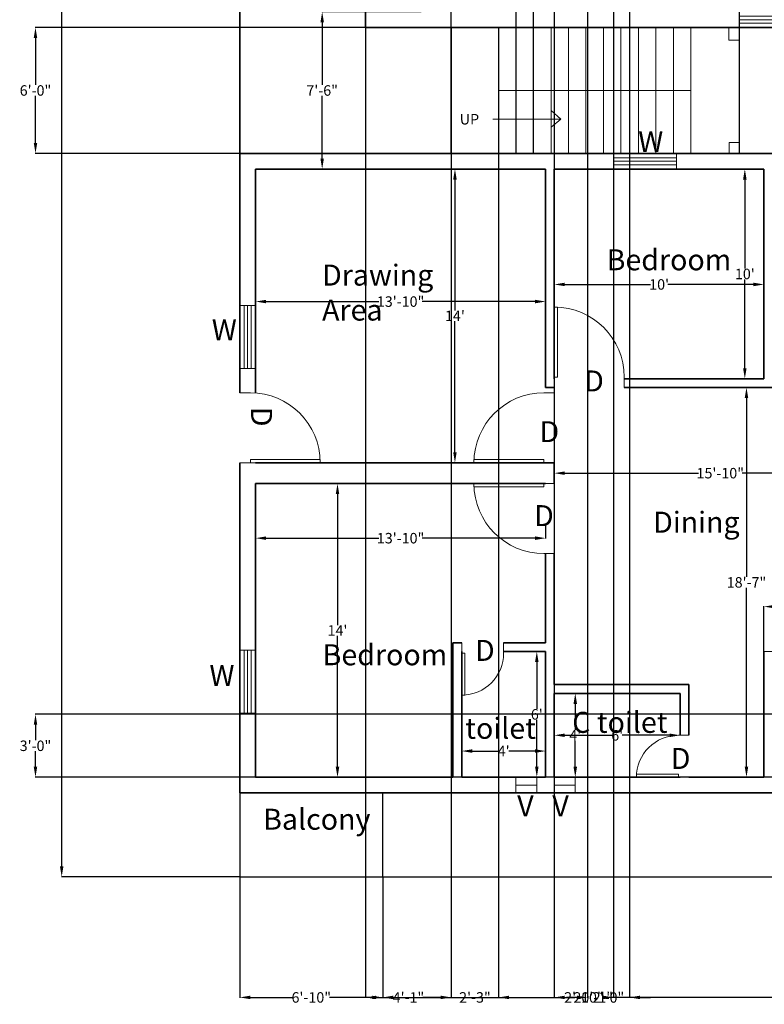
# Model space of a CAD drawing. Units: inches. Extents: x 1936 to 2761, y 1431 to 2889.
# Tile 1 of 6: x 1943 to 2369, y 1436 to 1999. Entities that reach past the tile are written whole.
import ezdxf

# ---------------------------------------------------------------- set-up
doc = ezdxf.new("R2010")
doc.units = ezdxf.units.IN
doc.header["$MEASUREMENT"] = 0
for name, color, linetype, lineweight in [('A-ANNO-DIMS', 172, 'Continuous', 13), ('A-ANNO-SYMB', 50, 'Continuous', 18), ('A-ANNO-TEXT', 50, 'Continuous', 18), ('A-AREA-IDEN', 50, 'Continuous', 18), ('A-FLOR-EDGE', 4, 'Continuous', 25), ('A-FLOR-FIXT', 8, 'Continuous', 18), ('A-GLAZ', 3, 'Continuous', 18), ('A-WALL', 4, 'Continuous', 35), ('doors', 10, 'Continuous', 18), ('stair', 94, 'Continuous', 18)]:
    doc.layers.add(name, color=color, linetype=linetype, lineweight=lineweight)
doc.styles.get("Standard").update_dxf_attribs({"font": 'arial.ttf'})
doc.dimstyles.get("Standard").update_dxf_attribs({"dimtxt": 6, "dimasz": 6, "dimexe": 0.18, "dimexo": 0.0625, "dimgap": 0.09, "dimtad": 0, "dimtih": 1, "dimtoh": 1, "dimdec": 0, "dimzin": 0, "dimdsep": 46, "dimlunit": 3, "dimtxsty": 'Standard', "dimcen": 0.09, "dimadec": 0, "dimazin": 0, "dimtfac": 1, "dimtdec": 0, "dimtofl": 0, "dimtmove": 0, "dimatfit": 3, "dimfxl": 1, "dimtolj": 1, "dimtzin": 0, "dimarcsym": 0})

# ---------------------------------------------------------------- blocks, each defined once
blk = doc.blocks.new('*U4')
for p, q in [((0, 0), (0, 6)), ((24, 0), (24, 6))]:
    blk.add_line(p, q)
blk.add_lwpolyline([(0, 0), (0, -24), (1.75, -24), (1.75, 0)], close=True)
blk.add_arc((0, 0), 24, 270, 0)
blk = doc.blocks.new('*U3')
for p, q in [((0, 0), (0, -6)), ((24, 0), (24, -6))]:
    blk.add_line(p, q)
blk.add_lwpolyline([(0, 0), (0, 24), (1.75, 24), (1.75, 0)], close=True)
blk.add_arc((0, 0), 24, 0, 90)
blk = doc.blocks.new('*U5')
for p, q in [((0, 0), (0, -6)), ((40, 0), (40, -6))]:
    blk.add_line(p, q)
blk.add_lwpolyline([(0, 0), (0, 40), (1.75, 40), (1.75, 0)], close=True)
blk.add_arc((0, 0), 40, 0, 90)
blk = doc.blocks.new('*U2')
for p, q in [((0, 0), (0, 6)), ((40, 0), (40, 6))]:
    blk.add_line(p, q)
blk.add_lwpolyline([(0, 0), (0, -40), (1.75, -40), (1.75, 0)], close=True)
blk.add_arc((0, 0), 40, 270, 360)
blk = doc.blocks.new('*D57')
at = {"layer": 'A-ANNO-DIMS', "color": 0, "lineweight": -2, "transparency": 16777216}
for p, q in [((2078.01, 1709.55), (2078.01, 1702.17)), ((2244.01, 1709.55), (2244.01, 1702.17)), ((2084.01, 1702.35), (2148.56, 1702.35)), ((2238.01, 1702.35), (2173.45, 1702.35))]:
    blk.add_line(p, q, dxfattribs=at)
at = {"layer": 'A-ANNO-DIMS', "color": 0, "transparency": 16777216}
for points in [[(2084.01, 1703.35), (2084.01, 1701.35), (2078.01, 1702.35)], [(2238.01, 1703.35), (2238.01, 1701.35), (2244.01, 1702.35)]]:
    blk.add_solid(points, dxfattribs=at)
at = {"layer": 'Defpoints', "color": 0, "transparency": 16777216}
for p in [(2078.01, 1709.61), (2244.01, 1709.61), (2244.01, 1702.35)]:
    blk.add_point(p, dxfattribs=at)
at = {"layer": 'A-ANNO-DIMS', "color": 0, "transparency": 16777216, "insert": (2161.01, 1702.35), "char_height": 6, "attachment_point": 5}
blk.add_mtext('\\A1;13\'-10"', dxfattribs=at)
blk = doc.blocks.new('*D58')
at = {"layer": 'A-ANNO-DIMS', "color": 0, "lineweight": -2, "transparency": 16777216}
for p, q in [((2124.95, 1733.55), (2125.07, 1733.55)), ((2124.89, 1727.55), (2124.89, 1652.65)), ((2124.89, 1571.55), (2124.89, 1646.45)), ((2124.95, 1565.55), (2125.07, 1565.55))]:
    blk.add_line(p, q, dxfattribs=at)
at = {"layer": 'A-ANNO-DIMS', "color": 0, "transparency": 16777216}
for points in [[(2123.89, 1727.55), (2125.89, 1727.55), (2124.89, 1733.55)], [(2123.89, 1571.55), (2125.89, 1571.55), (2124.89, 1565.55)]]:
    blk.add_solid(points, dxfattribs=at)
at = {"layer": 'Defpoints', "color": 0, "transparency": 16777216}
for p in [(2124.89, 1733.55), (2124.89, 1733.55), (2124.89, 1565.55)]:
    blk.add_point(p, dxfattribs=at)
at = {"layer": 'A-ANNO-DIMS', "color": 0, "transparency": 16777216, "insert": (2124.89, 1649.55), "char_height": 6, "attachment_point": 5}
blk.add_mtext("\\A1;14'", dxfattribs=at)
blk = doc.blocks.new('*D59')
at = {"layer": 'A-ANNO-DIMS', "color": 0, "lineweight": -2, "transparency": 16777216}
for p, q in [((2249.01, 1739.61), (2249.01, 1739.73)), ((2255.01, 1739.55), (2331.56, 1739.55)), ((2433.01, 1739.55), (2356.45, 1739.55)), ((2439.01, 1739.61), (2439.01, 1739.73))]:
    blk.add_line(p, q, dxfattribs=at)
at = {"layer": 'A-ANNO-DIMS', "color": 0, "transparency": 16777216}
for points in [[(2255.01, 1740.55), (2255.01, 1738.55), (2249.01, 1739.55)], [(2433.01, 1740.55), (2433.01, 1738.55), (2439.01, 1739.55)]]:
    blk.add_solid(points, dxfattribs=at)
at = {"layer": 'Defpoints', "color": 0, "transparency": 16777216}
for p in [(2249.01, 1739.55), (2439.01, 1739.55), (2439.01, 1739.55)]:
    blk.add_point(p, dxfattribs=at)
at = {"layer": 'A-ANNO-DIMS', "color": 0, "transparency": 16777216, "insert": (2344.01, 1739.55), "char_height": 6, "attachment_point": 5}
blk.add_mtext('\\A1;15\'-10"', dxfattribs=at)
blk = doc.blocks.new('*D60')
at = {"layer": 'A-ANNO-DIMS', "color": 0, "lineweight": -2, "transparency": 16777216}
for p, q in [((2347.57, 1788.55), (2359.19, 1788.55)), ((2359.01, 1782.55), (2359.01, 1680.2)), ((2359.01, 1571.55), (2359.01, 1673.9)), ((2347.57, 1565.55), (2359.19, 1565.55))]:
    blk.add_line(p, q, dxfattribs=at)
at = {"layer": 'A-ANNO-DIMS', "color": 0, "transparency": 16777216}
for points in [[(2358.01, 1782.55), (2360.01, 1782.55), (2359.01, 1788.55)], [(2358.01, 1571.55), (2360.01, 1571.55), (2359.01, 1565.55)]]:
    blk.add_solid(points, dxfattribs=at)
at = {"layer": 'Defpoints', "color": 0, "transparency": 16777216}
for p in [(2347.51, 1788.55), (2359.01, 1788.55), (2347.51, 1565.55)]:
    blk.add_point(p, dxfattribs=at)
at = {"layer": 'A-ANNO-DIMS', "color": 0, "transparency": 16777216, "insert": (2359.01, 1677.05), "char_height": 6, "attachment_point": 5}
blk.add_mtext('\\A1;18\'-7"', dxfattribs=at)
blk = doc.blocks.new('*D65')
at = {"layer": 'A-ANNO-DIMS', "color": 0, "lineweight": -2, "transparency": 16777216}
for p, q in [((2249.01, 1589.61), (2249.01, 1589.73)), ((2255.01, 1589.55), (2282.14, 1589.55)), ((2315.01, 1589.55), (2287.87, 1589.55)), ((2321.01, 1589.61), (2321.01, 1589.73))]:
    blk.add_line(p, q, dxfattribs=at)
at = {"layer": 'A-ANNO-DIMS', "color": 0, "transparency": 16777216}
for points in [[(2255.01, 1590.55), (2255.01, 1588.55), (2249.01, 1589.55)], [(2315.01, 1590.55), (2315.01, 1588.55), (2321.01, 1589.55)]]:
    blk.add_solid(points, dxfattribs=at)
at = {"layer": 'Defpoints', "color": 0, "transparency": 16777216}
for p in [(2249.01, 1589.55), (2321.01, 1589.55), (2321.01, 1589.55)]:
    blk.add_point(p, dxfattribs=at)
at = {"layer": 'A-ANNO-DIMS', "color": 0, "transparency": 16777216, "insert": (2285.01, 1589.55), "char_height": 6, "attachment_point": 5}
blk.add_mtext("\\A1;6'", dxfattribs=at)
blk = doc.blocks.new('*D66')
at = {"layer": 'A-ANNO-DIMS', "color": 0, "lineweight": -2, "transparency": 16777216}
for p, q in [((2261.07, 1613.55), (2261.19, 1613.55)), ((2261.01, 1607.55), (2261.01, 1592.64)), ((2261.01, 1571.55), (2261.01, 1586.46)), ((2261.07, 1565.55), (2261.19, 1565.55))]:
    blk.add_line(p, q, dxfattribs=at)
at = {"layer": 'A-ANNO-DIMS', "color": 0, "transparency": 16777216}
for points in [[(2260.01, 1607.55), (2262.01, 1607.55), (2261.01, 1613.55)], [(2260.01, 1571.55), (2262.01, 1571.55), (2261.01, 1565.55)]]:
    blk.add_solid(points, dxfattribs=at)
at = {"layer": 'Defpoints', "color": 0, "transparency": 16777216}
for p in [(2261.01, 1613.55), (2261.01, 1613.55), (2261.01, 1565.55)]:
    blk.add_point(p, dxfattribs=at)
at = {"layer": 'A-ANNO-DIMS', "color": 0, "transparency": 16777216, "insert": (2261.01, 1589.55), "char_height": 6, "attachment_point": 5}
blk.add_mtext("\\A1;4'", dxfattribs=at)
blk = doc.blocks.new('*D67')
at = {"layer": 'A-ANNO-DIMS', "color": 0, "lineweight": -2, "transparency": 16777216}
for p, q in [((2234.79, 1637.55), (2239.17, 1637.55)), ((2238.99, 1631.55), (2238.99, 1604.7)), ((2238.99, 1571.55), (2238.99, 1598.4)), ((2234.79, 1565.55), (2239.17, 1565.55))]:
    blk.add_line(p, q, dxfattribs=at)
at = {"layer": 'A-ANNO-DIMS', "color": 0, "transparency": 16777216}
for points in [[(2237.99, 1631.55), (2239.99, 1631.55), (2238.99, 1637.55)], [(2237.99, 1571.55), (2239.99, 1571.55), (2238.99, 1565.55)]]:
    blk.add_solid(points, dxfattribs=at)
at = {"layer": 'Defpoints', "color": 0, "transparency": 16777216}
for p in [(2234.73, 1637.55), (2238.99, 1637.55), (2234.73, 1565.55)]:
    blk.add_point(p, dxfattribs=at)
at = {"layer": 'A-ANNO-DIMS', "color": 0, "transparency": 16777216, "insert": (2238.99, 1601.55), "char_height": 6, "attachment_point": 5}
blk.add_mtext("\\A1;6'", dxfattribs=at)
blk = doc.blocks.new('*D68')
at = {"layer": 'A-ANNO-DIMS', "color": 0, "lineweight": -2, "transparency": 16777216}
for p, q in [((2196.01, 1580.6), (2196.01, 1580.72)), ((2202.01, 1580.54), (2217.03, 1580.54)), ((2238.01, 1580.54), (2222.98, 1580.54)), ((2244.01, 1580.6), (2244.01, 1580.72))]:
    blk.add_line(p, q, dxfattribs=at)
at = {"layer": 'A-ANNO-DIMS', "color": 0, "transparency": 16777216}
for points in [[(2202.01, 1581.54), (2202.01, 1579.54), (2196.01, 1580.54)], [(2238.01, 1581.54), (2238.01, 1579.54), (2244.01, 1580.54)]]:
    blk.add_solid(points, dxfattribs=at)
at = {"layer": 'Defpoints', "color": 0, "transparency": 16777216}
for p in [(2196.01, 1580.54), (2196.01, 1580.54), (2244.01, 1580.54)]:
    blk.add_point(p, dxfattribs=at)
at = {"layer": 'A-ANNO-DIMS', "color": 0, "transparency": 16777216, "insert": (2220.01, 1580.54), "char_height": 6, "attachment_point": 5}
blk.add_mtext("\\A1;4'", dxfattribs=at)
blk = doc.blocks.new('*D69')
at = {"layer": 'A-ANNO-DIMS', "color": 0, "lineweight": -2, "transparency": 16777216}
for p, q in [((2078.01, 1837.81), (2078.01, 1837.93)), ((2084.01, 1837.75), (2148.56, 1837.75)), ((2238.01, 1837.75), (2173.45, 1837.75)), ((2244.01, 1837.81), (2244.01, 1837.93))]:
    blk.add_line(p, q, dxfattribs=at)
at = {"layer": 'A-ANNO-DIMS', "color": 0, "transparency": 16777216}
for points in [[(2084.01, 1838.75), (2084.01, 1836.75), (2078.01, 1837.75)], [(2238.01, 1838.75), (2238.01, 1836.75), (2244.01, 1837.75)]]:
    blk.add_solid(points, dxfattribs=at)
at = {"layer": 'Defpoints', "color": 0, "transparency": 16777216}
for p in [(2078.01, 1837.75), (2244.01, 1837.75), (2244.01, 1837.75)]:
    blk.add_point(p, dxfattribs=at)
at = {"layer": 'A-ANNO-DIMS', "color": 0, "transparency": 16777216, "insert": (2161.01, 1837.75), "char_height": 6, "attachment_point": 5}
blk.add_mtext('\\A1;13\'-10"', dxfattribs=at)
blk = doc.blocks.new('*D70')
at = {"layer": 'A-ANNO-DIMS', "color": 0, "lineweight": -2, "transparency": 16777216}
for p, q in [((2187.65, 1913.55), (2192.3, 1913.55)), ((2192.12, 1907.55), (2192.12, 1832.65)), ((2192.12, 1751.55), (2192.12, 1826.45)), ((2187.65, 1745.55), (2192.3, 1745.55))]:
    blk.add_line(p, q, dxfattribs=at)
at = {"layer": 'A-ANNO-DIMS', "color": 0, "transparency": 16777216}
for points in [[(2191.12, 1907.55), (2193.12, 1907.55), (2192.12, 1913.55)], [(2191.12, 1751.55), (2193.12, 1751.55), (2192.12, 1745.55)]]:
    blk.add_solid(points, dxfattribs=at)
at = {"layer": 'Defpoints', "color": 0, "transparency": 16777216}
for p in [(2187.59, 1913.55), (2192.12, 1913.55), (2187.59, 1745.55)]:
    blk.add_point(p, dxfattribs=at)
at = {"layer": 'A-ANNO-DIMS', "color": 0, "transparency": 16777216, "insert": (2192.12, 1829.55), "char_height": 6, "attachment_point": 5}
blk.add_mtext("\\A1;14'", dxfattribs=at)
blk = doc.blocks.new('*D71')
at = {"layer": 'A-ANNO-DIMS', "color": 0, "lineweight": -2, "transparency": 16777216}
for p, q in [((2249.01, 1853.49), (2249.01, 1847.37)), ((2369.01, 1853.49), (2369.01, 1847.37)), ((2255.01, 1847.55), (2304.11, 1847.55)), ((2363.01, 1847.55), (2313.91, 1847.55))]:
    blk.add_line(p, q, dxfattribs=at)
at = {"layer": 'A-ANNO-DIMS', "color": 0, "transparency": 16777216}
for points in [[(2255.01, 1848.55), (2255.01, 1846.55), (2249.01, 1847.55)], [(2363.01, 1848.55), (2363.01, 1846.55), (2369.01, 1847.55)]]:
    blk.add_solid(points, dxfattribs=at)
at = {"layer": 'Defpoints', "color": 0, "transparency": 16777216}
for p in [(2249.01, 1853.55), (2369.01, 1853.55), (2249.01, 1847.55)]:
    blk.add_point(p, dxfattribs=at)
at = {"layer": 'A-ANNO-DIMS', "color": 0, "transparency": 16777216, "insert": (2309.01, 1847.55), "char_height": 6, "attachment_point": 5}
blk.add_mtext("\\A1;10'", dxfattribs=at)
blk = doc.blocks.new('*D72')
at = {"layer": 'A-ANNO-DIMS', "color": 0, "lineweight": -2, "transparency": 16777216}
for p, q in [((2354.08, 1913.55), (2358.25, 1913.55)), ((2358.07, 1907.55), (2358.07, 1856.7)), ((2358.07, 1799.55), (2358.07, 1850.4)), ((2354.08, 1793.55), (2358.25, 1793.55))]:
    blk.add_line(p, q, dxfattribs=at)
at = {"layer": 'A-ANNO-DIMS', "color": 0, "transparency": 16777216}
for points in [[(2357.07, 1907.55), (2359.07, 1907.55), (2358.07, 1913.55)], [(2357.07, 1799.55), (2359.07, 1799.55), (2358.07, 1793.55)]]:
    blk.add_solid(points, dxfattribs=at)
at = {"layer": 'Defpoints', "color": 0, "transparency": 16777216}
for p in [(2354.02, 1913.55), (2358.07, 1913.55), (2354.02, 1793.55)]:
    blk.add_point(p, dxfattribs=at)
at = {"layer": 'A-ANNO-DIMS', "color": 0, "transparency": 16777216, "insert": (2358.07, 1853.55), "char_height": 6, "attachment_point": 5}
blk.add_mtext("\\A1;10'", dxfattribs=at)
blk = doc.blocks.new('*U55')
for p, q in [((-40, 0), (-40, 6)), ((0, 0), (0, 6))]:
    blk.add_line(p, q)
blk.add_lwpolyline([(0, 0), (0, -40), (-1.75, -40), (-1.75, 0)], close=True)
blk.add_arc((0, 0), 40, 180, 270)
blk = doc.blocks.new('*D76')
at = {"layer": 'A-ANNO-DIMS', "color": 0, "lineweight": -2, "transparency": 16777216}
for p, q in [((2068.94, 2816.55), (1966.82, 2816.55)), ((1967, 2810.55), (1967, 2168.77)), ((1967, 1514.55), (1967, 2156.33)), ((2068.94, 1508.55), (1966.82, 1508.55))]:
    blk.add_line(p, q, dxfattribs=at)
at = {"layer": 'A-ANNO-DIMS', "color": 0, "transparency": 16777216}
for points in [[(1966, 2810.55), (1968, 2810.55), (1967, 2816.55)], [(1966, 1514.55), (1968, 1514.55), (1967, 1508.55)]]:
    blk.add_solid(points, dxfattribs=at)
at = {"layer": 'Defpoints', "color": 0, "transparency": 16777216}
for p in [(2069.01, 2816.55), (1967, 1508.55), (2069.01, 1508.55)]:
    blk.add_point(p, dxfattribs=at)
at = {"layer": 'A-ANNO-DIMS', "color": 0, "transparency": 16777216, "insert": (1967, 2162.55), "char_height": 6, "attachment_point": 5}
blk.add_mtext("\\A1;{\\H2x;109'}", dxfattribs=at)
blk = doc.blocks.new('*D77')
at = {"layer": 'A-ANNO-DIMS', "color": 0, "lineweight": -2, "transparency": 16777216}
for p, q in [((2172.87, 2003.55), (2115.94, 2003.55)), ((2116.12, 1997.55), (2116.12, 1961.7)), ((2116.12, 1919.55), (2116.12, 1955.4)), ((2160.94, 1913.55), (2115.94, 1913.55))]:
    blk.add_line(p, q, dxfattribs=at)
at = {"layer": 'A-ANNO-DIMS', "color": 0, "transparency": 16777216}
for points in [[(2115.12, 1997.55), (2117.12, 1997.55), (2116.12, 2003.55)], [(2115.12, 1919.55), (2117.12, 1919.55), (2116.12, 1913.55)]]:
    blk.add_solid(points, dxfattribs=at)
at = {"layer": 'Defpoints', "color": 0, "transparency": 16777216}
for p in [(2172.93, 2003.55), (2116.12, 1913.55), (2161.01, 1913.55)]:
    blk.add_point(p, dxfattribs=at)
at = {"layer": 'A-ANNO-DIMS', "color": 0, "transparency": 16777216, "insert": (2116.12, 1958.55), "char_height": 6, "attachment_point": 5}
blk.add_mtext('\\A1;7\'-6"', dxfattribs=at)
blk = doc.blocks.new('WIN-36')
for p, q in [((0, 9), (0, 0)), ((36, 6.5), (0, 6.5)), ((36, 9), (36, 0)), ((36, 4.5), (0, 4.5)), ((36, 2.5), (0, 2.5))]:
    blk.add_line(p, q)
blk = doc.blocks.new('VENT-12')
for p, q in [((0, 0), (0, 9)), ((12, 0), (12, 9)), ((0, 4.5), (12, 4.5))]:
    blk.add_line(p, q)
blk = doc.blocks.new('COUNTER-KITCHEN-U')
for p, q in [((41, 36), (41, 0)), ((41, 36), (135, 36)), ((135, 36), (135, 0)), ((0, 0), (41, 0)), ((135, 0), (171, 0))]:
    blk.add_line(p, q)
blk = doc.blocks.new('*D93')
at = {"layer": 'A-ANNO-DIMS', "color": 0, "lineweight": -2, "transparency": 16777216}
for p, q in [((2369.01, 1637.61), (2369.01, 1663.38)), ((2375.01, 1663.2), (2411.95, 1663.2)), ((2534.01, 1663.2), (2497.06, 1663.2)), ((2540.01, 1637.61), (2540.01, 1663.38))]:
    blk.add_line(p, q, dxfattribs=at)
at = {"layer": 'A-ANNO-DIMS', "color": 0, "transparency": 16777216}
for points in [[(2375.01, 1664.2), (2375.01, 1662.2), (2369.01, 1663.2)], [(2534.01, 1664.2), (2534.01, 1662.2), (2540.01, 1663.2)]]:
    blk.add_solid(points, dxfattribs=at)
at = {"layer": 'Defpoints', "color": 0, "transparency": 16777216}
for p in [(2540.01, 1663.2), (2369.01, 1637.55), (2540.01, 1637.55)]:
    blk.add_point(p, dxfattribs=at)
at = {"layer": 'A-ANNO-DIMS', "color": 0, "transparency": 16777216, "insert": (2454.51, 1663.2), "char_height": 6, "attachment_point": 5}
blk.add_mtext('\\A1;COUNTER 14\'-3" TYP.', dxfattribs=at)
blk = doc.blocks.new('*D100')
at = {"layer": 'A-ANNO-DIMS', "color": 0, "lineweight": -2, "transparency": 16777216}
for p, q in [((2069.01, 1508.49), (2069.01, 1439.37)), ((2150.78, 1508.49), (2150.78, 1439.37)), ((2075.01, 1439.55), (2099.48, 1439.55)), ((2144.78, 1439.55), (2120.31, 1439.55))]:
    blk.add_line(p, q, dxfattribs=at)
at = {"layer": 'A-ANNO-DIMS', "color": 0, "transparency": 16777216}
for points in [[(2075.01, 1440.55), (2075.01, 1438.55), (2069.01, 1439.55)], [(2144.78, 1440.55), (2144.78, 1438.55), (2150.78, 1439.55)]]:
    blk.add_solid(points, dxfattribs=at)
at = {"layer": 'Defpoints', "color": 0, "transparency": 16777216}
for p in [(2069.01, 1508.55), (2150.78, 1508.55), (2150.78, 1439.55)]:
    blk.add_point(p, dxfattribs=at)
at = {"layer": 'A-ANNO-DIMS', "color": 0, "transparency": 16777216, "insert": (2109.89, 1439.55), "char_height": 6, "attachment_point": 5}
blk.add_mtext('\\A1;6\'-10"', dxfattribs=at)
blk = doc.blocks.new('*D102')
at = {"layer": 'A-ANNO-DIMS', "color": 0, "lineweight": -2, "transparency": 16777216}
for p, q in [((2150.85, 1556.55), (2738.19, 1556.55)), ((2738.01, 1550.55), (2738.01, 1535.7)), ((2738.01, 1514.55), (2738.01, 1529.4)), ((2150.85, 1508.55), (2738.19, 1508.55))]:
    blk.add_line(p, q, dxfattribs=at)
at = {"layer": 'A-ANNO-DIMS', "color": 0, "transparency": 16777216}
for points in [[(2737.01, 1550.55), (2739.01, 1550.55), (2738.01, 1556.55)], [(2737.01, 1514.55), (2739.01, 1514.55), (2738.01, 1508.55)]]:
    blk.add_solid(points, dxfattribs=at)
at = {"layer": 'Defpoints', "color": 0, "transparency": 16777216}
for p in [(2150.78, 1556.55), (2738.01, 1556.55), (2150.78, 1508.55)]:
    blk.add_point(p, dxfattribs=at)
at = {"layer": 'A-ANNO-DIMS', "color": 0, "transparency": 16777216, "insert": (2738.01, 1532.55), "char_height": 6, "attachment_point": 5}
blk.add_mtext('\\A1;4\'-0"', dxfattribs=at)
blk = doc.blocks.new('*D103')
at = {"layer": 'A-ANNO-DIMS', "color": 0, "lineweight": -2, "transparency": 16777216}
for p, q in [((2150.78, 1508.49), (2150.78, 1439.37)), ((2391.78, 1508.49), (2391.78, 1439.37)), ((2156.78, 1439.55), (2260.84, 1439.55)), ((2385.78, 1439.55), (2281.73, 1439.55))]:
    blk.add_line(p, q, dxfattribs=at)
at = {"layer": 'A-ANNO-DIMS', "color": 0, "transparency": 16777216}
for points in [[(2156.78, 1440.55), (2156.78, 1438.55), (2150.78, 1439.55)], [(2385.78, 1440.55), (2385.78, 1438.55), (2391.78, 1439.55)]]:
    blk.add_solid(points, dxfattribs=at)
at = {"layer": 'Defpoints', "color": 0, "transparency": 16777216}
for p in [(2150.78, 1508.55), (2391.78, 1508.55), (2391.78, 1439.55)]:
    blk.add_point(p, dxfattribs=at)
at = {"layer": 'A-ANNO-DIMS', "color": 0, "transparency": 16777216, "insert": (2271.28, 1439.55), "char_height": 6, "attachment_point": 5}
blk.add_mtext('\\A1;20\'-1"', dxfattribs=at)
blk = doc.blocks.new('*D104')
at = {"layer": 'A-ANNO-DIMS', "color": 0, "lineweight": -2, "transparency": 16777216}
for p, q in [((2190.01, 1922.61), (2190.01, 2885.73)), ((2196.01, 2885.55), (2262.35, 2885.55)), ((2348.92, 2885.55), (2282.58, 2885.55)), ((2354.92, 1922.61), (2354.92, 2885.73))]:
    blk.add_line(p, q, dxfattribs=at)
at = {"layer": 'A-ANNO-DIMS', "color": 0, "transparency": 16777216}
for points in [[(2196.01, 2886.55), (2196.01, 2884.55), (2190.01, 2885.55)], [(2348.92, 2886.55), (2348.92, 2884.55), (2354.92, 2885.55)]]:
    blk.add_solid(points, dxfattribs=at)
at = {"layer": 'Defpoints', "color": 0, "transparency": 16777216}
for p in [(2354.92, 2885.55), (2190.01, 1922.55), (2354.92, 1922.55)]:
    blk.add_point(p, dxfattribs=at)
at = {"layer": 'A-ANNO-DIMS', "color": 0, "transparency": 16777216, "insert": (2272.46, 2885.55), "char_height": 6, "attachment_point": 5}
blk.add_mtext('\\A1;13\'-9"', dxfattribs=at)
blk = doc.blocks.new('*D105')
at = {"layer": 'A-ANNO-DIMS', "color": 0, "lineweight": -2, "transparency": 16777216}
for p, q in [((2189.94, 1994.55), (1951.83, 1994.55)), ((1952.01, 1988.55), (1952.01, 1961.7)), ((1952.01, 1928.55), (1952.01, 1955.4)), ((2189.94, 1922.55), (1951.83, 1922.55))]:
    blk.add_line(p, q, dxfattribs=at)
at = {"layer": 'A-ANNO-DIMS', "color": 0, "transparency": 16777216}
for points in [[(1951.01, 1988.55), (1953.01, 1988.55), (1952.01, 1994.55)], [(1951.01, 1928.55), (1953.01, 1928.55), (1952.01, 1922.55)]]:
    blk.add_solid(points, dxfattribs=at)
at = {"layer": 'Defpoints', "color": 0, "transparency": 16777216}
for p in [(1952.01, 1994.55), (2190.01, 1994.55), (2190.01, 1922.55)]:
    blk.add_point(p, dxfattribs=at)
at = {"layer": 'A-ANNO-DIMS', "color": 0, "transparency": 16777216, "insert": (1952.01, 1958.55), "char_height": 6, "attachment_point": 5}
blk.add_mtext('\\A1;6\'-0"', dxfattribs=at)
blk = doc.blocks.new('*D106')
at = {"layer": 'A-ANNO-DIMS', "color": 0, "lineweight": -2, "transparency": 16777216}
for p, q in [((2141.01, 1994.49), (2141.01, 1439.37)), ((2190.01, 1994.49), (2190.01, 1439.37)), ((2147.01, 1439.55), (2157.32, 1439.55)), ((2184.01, 1439.55), (2173.69, 1439.55))]:
    blk.add_line(p, q, dxfattribs=at)
at = {"layer": 'A-ANNO-DIMS', "color": 0, "transparency": 16777216}
for points in [[(2147.01, 1440.55), (2147.01, 1438.55), (2141.01, 1439.55)], [(2184.01, 1440.55), (2184.01, 1438.55), (2190.01, 1439.55)]]:
    blk.add_solid(points, dxfattribs=at)
at = {"layer": 'Defpoints', "color": 0, "transparency": 16777216}
for p in [(2141.01, 1994.55), (2190.01, 1994.55), (2141.01, 1439.55)]:
    blk.add_point(p, dxfattribs=at)
at = {"layer": 'A-ANNO-DIMS', "color": 0, "transparency": 16777216, "insert": (2165.51, 1439.55), "char_height": 6, "attachment_point": 5}
blk.add_mtext('\\A1;4\'-1"', dxfattribs=at)
blk = doc.blocks.new('*D107')
at = {"layer": 'A-ANNO-DIMS', "color": 0, "lineweight": -2, "transparency": 16777216}
for p, q in [((2221.14, 2885.55), (2215.14, 2885.55)), ((2227.14, 1922.61), (2227.14, 2885.73)), ((2237.14, 1922.61), (2237.14, 2885.73)), ((2243.14, 2885.55), (2249.14, 2885.55))]:
    blk.add_line(p, q, dxfattribs=at)
at = {"layer": 'A-ANNO-DIMS', "color": 0, "transparency": 16777216}
for points in [[(2221.14, 2886.55), (2221.14, 2884.55), (2227.14, 2885.55)], [(2243.14, 2886.55), (2243.14, 2884.55), (2237.14, 2885.55)]]:
    blk.add_solid(points, dxfattribs=at)
at = {"layer": 'Defpoints', "color": 0, "transparency": 16777216}
for p in [(2237.14, 2885.55), (2227.14, 1922.55), (2237.14, 1922.55)]:
    blk.add_point(p, dxfattribs=at)
at = {"layer": 'A-ANNO-DIMS', "color": 0, "transparency": 16777216, "insert": (2259.54, 2885.55), "char_height": 6, "attachment_point": 5}
blk.add_mtext('\\A1;0\'-10"', dxfattribs=at)
blk = doc.blocks.new('*D110')
at = {"layer": 'A-ANNO-DIMS', "color": 0, "lineweight": -2, "transparency": 16777216}
for p, q in [((2268.006183, 2279.486911), (2268.006183, 1439.369411)), ((2292.006183, 2279.486911), (2292.006183, 1439.369411)), ((2262.006183, 1439.549411), (2256.006183, 1439.549411)), ((2298.006183, 1439.549411), (2304.006183, 1439.549411))]:
    blk.add_line(p, q, dxfattribs=at)
at = {"layer": 'A-ANNO-DIMS', "color": 0, "transparency": 16777216}
for points in [[(2262.006183, 1440.549411), (2262.006183, 1438.549411), (2268.006183, 1439.549411)], [(2298.006183, 1440.549411), (2298.006183, 1438.549411), (2292.006183, 1439.549411)]]:
    blk.add_solid(points, dxfattribs=at)
at = {"layer": 'Defpoints', "color": 0, "transparency": 16777216}
for p in [(2268.006183, 2279.549411), (2292.006183, 2279.549411), (2292.006183, 1439.549411)]:
    blk.add_point(p, dxfattribs=at)
at = {"layer": 'A-ANNO-DIMS', "color": 0, "transparency": 16777216, "insert": (2280.006183, 1439.549411), "char_height": 6, "attachment_point": 5}
blk.add_mtext('\\A1;2\'-0"', dxfattribs=at)
blk = doc.blocks.new('*D117')
at = {"layer": 'A-ANNO-DIMS', "color": 0, "lineweight": -2, "transparency": 16777216}
for p, q in [((2409.94, 1601.55), (1951.83, 1601.55)), ((1952.01, 1595.55), (1952.01, 1586.7)), ((1952.01, 1571.55), (1952.01, 1580.39)), ((2373.94, 1565.55), (1951.83, 1565.55))]:
    blk.add_line(p, q, dxfattribs=at)
at = {"layer": 'A-ANNO-DIMS', "color": 0, "transparency": 16777216}
for points in [[(1951.01, 1595.55), (1953.01, 1595.55), (1952.01, 1601.55)], [(1951.01, 1571.55), (1953.01, 1571.55), (1952.01, 1565.55)]]:
    blk.add_solid(points, dxfattribs=at)
at = {"layer": 'Defpoints', "color": 0, "transparency": 16777216}
for p in [(1952.01, 1601.55), (2410.01, 1601.55), (2374.01, 1565.55)]:
    blk.add_point(p, dxfattribs=at)
at = {"layer": 'A-ANNO-DIMS', "color": 0, "transparency": 16777216, "insert": (1952.01, 1583.55), "char_height": 6, "attachment_point": 5}
blk.add_mtext('\\A1;3\'-0"', dxfattribs=at)
blk = doc.blocks.new('*D120')
at = {"layer": 'A-ANNO-DIMS', "color": 0, "lineweight": -2, "transparency": 16777216}
for p, q in [((2249.01, 2459.49), (2249.01, 1439.37)), ((2282.92, 2450.49), (2282.92, 1439.37)), ((2255.01, 1439.55), (2255.52, 1439.55)), ((2276.92, 1439.55), (2276.41, 1439.55))]:
    blk.add_line(p, q, dxfattribs=at)
at = {"layer": 'A-ANNO-DIMS', "color": 0, "transparency": 16777216}
for points in [[(2255.01, 1440.55), (2255.01, 1438.55), (2249.01, 1439.55)], [(2276.92, 1440.55), (2276.92, 1438.55), (2282.92, 1439.55)]]:
    blk.add_solid(points, dxfattribs=at)
at = {"layer": 'Defpoints', "color": 0, "transparency": 16777216}
for p in [(2249.01, 2459.55), (2282.92, 2450.55), (2282.92, 1439.55)]:
    blk.add_point(p, dxfattribs=at)
at = {"layer": 'A-ANNO-DIMS', "color": 0, "transparency": 16777216, "insert": (2265.96, 1439.55), "char_height": 6, "attachment_point": 5}
blk.add_mtext('\\A1;2\'-10"', dxfattribs=at)
blk = doc.blocks.new('*D121')
at = {"layer": 'A-ANNO-DIMS', "color": 0, "lineweight": -2, "transparency": 16777216}
for p, q in [((2190.01, 1994.49), (2190.01, 1439.37)), ((2217.14, 1994.49), (2217.14, 1439.37)), ((2184.01, 1439.55), (2178.01, 1439.55)), ((2223.14, 1439.55), (2229.14, 1439.55))]:
    blk.add_line(p, q, dxfattribs=at)
at = {"layer": 'A-ANNO-DIMS', "color": 0, "transparency": 16777216}
for points in [[(2184.01, 1440.55), (2184.01, 1438.55), (2190.01, 1439.55)], [(2223.14, 1440.55), (2223.14, 1438.55), (2217.14, 1439.55)]]:
    blk.add_solid(points, dxfattribs=at)
at = {"layer": 'Defpoints', "color": 0, "transparency": 16777216}
for p in [(2190.01, 1994.55), (2217.14, 1994.55), (2217.14, 1439.55)]:
    blk.add_point(p, dxfattribs=at)
at = {"layer": 'A-ANNO-DIMS', "color": 0, "transparency": 16777216, "insert": (2203.57, 1439.55), "char_height": 6, "attachment_point": 5}
blk.add_mtext('\\A1;2\'-3"', dxfattribs=at)

msp = doc.modelspace()

# ---------------------------------------------------------------- linework, layer by layer
at = {"layer": 'A-ANNO-SYMB'}
for p, q in [((2252.69, 1942.1), (2247.14, 1947.06)), ((2247.14, 1947.06), (2247.14, 1937.64)), ((2213.74, 1942.1), (2252.69, 1942.1)), ((2247.14, 1937.64), (2252.69, 1942.1))]:
    msp.add_line(p, q, dxfattribs=at)
at = {"layer": 'A-FLOR-EDGE'}
for p, q in [((2069.01, 1556.55), (2069.01, 1508.55)), ((2150.78, 1508.55), (2150.78, 1556.55)), ((2069.01, 1508.55), (2150.78, 1508.55))]:
    msp.add_line(p, q, dxfattribs=at)
at = {"layer": 'A-WALL'}
for p, q in [((2069.01, 1867.87), (2069.01, 2639.55)), ((2141.01, 1994.55), (2141.01, 2131.55)), ((2621.01, 1994.55), (2141.01, 1994.55)), ((2150.01, 1994.55), (2141.01, 1994.55)), ((2549.01, 1922.55), (2069.01, 1922.55)), ((2078.01, 1922.55), (2069.01, 1922.55)), ((2069.01, 1922.55), (2069.01, 1785.55)), ((2244.01, 1913.55), (2078.01, 1913.55)), ((2078.01, 1913.55), (2078.01, 1785.44)), ((2244.01, 1913.55), (2244.01, 1788.55)), ((2369.01, 1913.55), (2249.01, 1913.55)), ((2249.01, 1913.55), (2249.01, 1793.55)), ((2369.01, 1793.55), (2369.01, 1913.55)), ((2369.01, 1793.55), (2289.01, 1793.55)), ((2249.01, 1788.55), (2244.01, 1788.55)), ((2374.01, 1788.55), (2289.01, 1788.55)), ((2069.01, 1745.55), (2069.01, 1556.55)), ((2249.01, 1745.55), (2078.01, 1745.55)), ((2249.01, 1745.55), (2249.01, 1733.55)), ((2078.01, 1733.55), (2078.01, 1565.55)), ((2078.01, 1733.55), (2244.01, 1733.55)), ((2244.01, 1693.55), (2244.01, 1642.55)), ((2249.01, 1693.55), (2249.01, 1618.55)), ((2191.01, 1642.55), (2191.01, 1565.55)), ((2191.01, 1642.55), (2196.01, 1642.55)), ((2220.01, 1642.55), (2244.01, 1642.55)), ((2196.01, 1637.55), (2196.01, 1565.55)), ((2220.01, 1637.55), (2244.01, 1637.55)), ((2244.01, 1637.55), (2244.01, 1565.55)), ((2369.01, 1565.55), (2369.01, 1637.55)), ((2249.01, 1618.55), (2326.01, 1618.55)), ((2326.01, 1618.55), (2326.01, 1589.55)), ((2249.01, 1613.55), (2249.01, 1565.55)), ((2249.01, 1613.55), (2321.01, 1613.55)), ((2321.01, 1613.55), (2321.01, 1589.55)), ((2078.01, 1565.55), (2191.01, 1565.55)), ((2196.01, 1565.55), (2244.01, 1565.55)), ((2249.01, 1565.55), (2321.01, 1565.55)), ((2326.01, 1565.55), (2369.01, 1565.55)), ((2069.01, 1556.55), (2597.01, 1556.55))]:
    msp.add_line(p, q, dxfattribs=at)
at = {"layer": 'doors'}
for p, q in [((2249.01, 1788.55), (2249.01, 1793.55)), ((2289.01, 1788.55), (2289.01, 1793.55)), ((2078.01, 1745.55), (2069.01, 1745.55)), ((2244.01, 1733.55), (2249.01, 1733.55)), ((2244.01, 1693.55), (2249.01, 1693.55)), ((2196.01, 1637.55), (2196.01, 1642.55)), ((2220.01, 1637.55), (2220.01, 1642.55)), ((2326.01, 1589.55), (2321.01, 1589.55)), ((2326.01, 1565.55), (2321.01, 1565.55))]:
    msp.add_line(p, q, dxfattribs=at)
at = {"layer": 'stair'}
for p, q in [((2190.01, 1994.55), (2190.01, 1922.55)), ((2217.14, 1994.55), (2217.14, 1922.55)), ((2227.14, 1994.55), (2227.14, 1922.55)), ((2237.14, 1994.55), (2237.14, 1922.55)), ((2247.14, 1994.55), (2247.14, 1922.55)), ((2257.14, 1994.55), (2257.14, 1922.55)), ((2267.14, 1994.55), (2267.14, 1922.55)), ((2277.14, 1994.55), (2277.14, 1922.55)), ((2287.14, 1994.55), (2287.14, 1922.55)), ((2297.14, 1994.55), (2297.14, 1922.55)), ((2307.14, 1994.55), (2307.14, 1922.55)), ((2317.14, 1994.55), (2317.14, 1922.55)), ((2327.14, 1994.55), (2327.14, 1922.55)), ((2354.92, 1994.55), (2354.92, 1922.55)), ((2327.14, 1958.55), (2217.14, 1958.55)), ((2354.92, 1922.55), (2069.01, 1922.55))]:
    msp.add_line(p, q, dxfattribs=at)
for points in [[(2354.92, 1994.55), (2348.85, 1994.55), (2348.85, 1987.36), (2354.92, 1987.36)], [(2354.92, 1922.55), (2349.1, 1922.55), (2349.1, 1928.72), (2354.92, 1928.72)]]:
    msp.add_lwpolyline(points, close=True, dxfattribs=at)

# ---------------------------------------------------------------- block references
at = {"layer": 'A-FLOR-FIXT', "extrusion": (0, 0, -1), "zscale": -1, "rotation": 180}
msp.add_blockref('COUNTER-KITCHEN-U', (-2369.01, 1637.55), dxfattribs=at)
at = {"layer": 'A-GLAZ'}
for name, p in [('WIN-36', (2354.92, 1994.55)), ('WIN-36', (2282.92, 1913.55)), ('VENT-12', (2227.01, 1556.55))]:
    msp.add_blockref(name, p, dxfattribs=at)
for name, p, rotation in [('WIN-36', (2077.91, 1799.44), 89.99999999999744), ('WIN-36', (2077.91, 1602.21), 89.99999999999763), ('VENT-12', (2261.01, 1565.55), 180)]:
    msp.add_blockref(name, p, dxfattribs=dict(at, rotation=rotation))
at = {"layer": 'doors', "xscale": -1}
for name, p, rotation in [('*U2', (2249.01, 1794.55), 180), ('*U55', (2075.01, 1745.55), 90), ('*U5', (2243.01, 1733.55), 90), ('*U3', (2196.01, 1636.55), 180), ('*U4', (2320.01, 1565.55), 270)]:
    msp.add_blockref(name, p, dxfattribs=dict(at, rotation=rotation))
at = {"layer": 'doors', "rotation": 90.00000000000003}
msp.add_blockref('*U5', (2243.01, 1745.55), dxfattribs=at)

# ---------------------------------------------------------------- texts
at = {"layer": 'A-ANNO-TEXT'}
for s, width, heights, insert, char_height, attachment_point in [('UP', 6.6996, [0], (2194.88, 1945.08), 6, 1), ('W', 7.8209, [0.2], (2297.01, 1923.25), 12, 7), ('W', 7.8209, [0.2], (2052.91, 1815.62), 12, 7), ('D', 28.2371, [0.2], (2266.1, 1786.32), 12, 7), ('D', 28.2371, [0.2], (2240.54, 1757.3), 12, 7), ('D', 28.2371, [0.2], (2237.43, 1709.25), 12, 7), ('D', 28.2371, [0.2], (2203.61, 1632.12), 12, 7), ('W', 7.8209, [0.2], (2051.56, 1617.84), 12, 7), ('D', 28.2371, [0.2], (2315.67, 1570.28), 12, 7), ('V', 13.1151, [0], (2227.76, 1543.19), 12, 7), ('V', 13.1151, [0], (2247.86, 1543.11), 12, 7)]:
    msp.add_mtext_dynamic_manual_height_columns(s, width=width, gutter_width=1, heights=heights, dxfattribs=dict(at, insert=insert, char_height=char_height, attachment_point=attachment_point))
at = {"layer": 'A-ANNO-TEXT', "insert": (2087.4, 1766.22), "char_height": 12, "attachment_point": 3, "rotation": 270}
msp.add_mtext_dynamic_manual_height_columns('D', width=28.2371, gutter_width=1, heights=[0.2], dxfattribs=at)
at = {"layer": 'A-AREA-IDEN', "char_height": 12}
for s, insert, attachment_point in [('Bedroom', (2278.96, 1855.65), 7), ('Drawing Area', (2116.07, 1826.88), 7), ('Dining', (2305.61, 1705.5), 7), ('Bedroom', (2116.37, 1629.62), 7), ('toilet', (2198.01, 1587.55), 7), ('C toilet', (2259.23, 1590.95), 7), ('Balcony', (2082.33, 1547.53), 1)]:
    msp.add_mtext_dynamic_manual_height_columns(s, width=55.7076, gutter_width=1, heights=[0], dxfattribs=dict(at, insert=insert, attachment_point=attachment_point))

# ---------------------------------------------------------------- dimensions: what is measured, and where the dimension line sits
at = {"layer": 'A-ANNO-DIMS'}
for base, p1, p2, override, picture, middle in [((2354.92, 2885.55), (2190.01, 1922.55), (2354.92, 1922.55), {"dimdec": 1, "dimlfac": 1, "dimrnd": 0, "dimzin": 1, "dimdsep": 46, "dimlunit": 4, "dimfrac": 2}, '*D104', (2272.46, 2885.55)), ((2237.14, 2885.55), (2227.14, 1922.55), (2237.14, 1922.55), {"dimdec": 1, "dimlfac": 1, "dimrnd": 0, "dimzin": 1, "dimdsep": 46, "dimlunit": 4, "dimfrac": 2}, '*D107', (2259.54, 2885.55)), ((2282.92, 1439.55), (2249.01, 2459.55), (2282.92, 2450.55), {"dimdec": 1, "dimlfac": 1, "dimrnd": 0, "dimzin": 1, "dimdsep": 46, "dimlunit": 4, "dimfrac": 2}, '*D120', (2265.96, 1439.55)), ((2292.01, 1439.55), (2268.01, 2279.55), (2292.01, 2279.55), {"dimdec": 1, "dimlfac": 1, "dimrnd": 0, "dimzin": 1, "dimdsep": 46, "dimlunit": 4, "dimfrac": 2}, '*D110', (2280.01, 1439.55)), ((2141.01, 1439.55), (2190.01, 1994.55), (2141.01, 1994.55), {"dimdec": 1, "dimlfac": 1, "dimrnd": 0, "dimzin": 1, "dimdsep": 46, "dimlunit": 4, "dimfrac": 2}, '*D106', (2165.51, 1439.55)), ((2217.14, 1439.55), (2190.01, 1994.55), (2217.14, 1994.55), {"dimdec": 1, "dimlfac": 1, "dimrnd": 0, "dimzin": 1, "dimdsep": 46, "dimlunit": 4, "dimfrac": 2}, '*D121', (2203.57, 1439.55)), ((2249.01, 1847.55), (2369.01, 1853.55), (2249.01, 1853.55), {"dimclrd": 0, "dimclre": 0, "dimclrt": 0}, '*D71', (2309.01, 1847.55)), ((2244.01, 1837.75), (2078.01, 1837.75), (2244.01, 1837.75), {"dimclrd": 0, "dimclre": 0, "dimclrt": 0}, '*D69', (2161.01, 1837.75)), ((2439.01, 1739.55), (2249.01, 1739.55), (2439.01, 1739.55), {"dimclrd": 0, "dimclre": 0, "dimclrt": 0}, '*D59', (2344.01, 1739.55)), ((2244.01, 1702.35), (2078.01, 1709.61), (2244.01, 1709.61), {"dimclrd": 0, "dimclre": 0, "dimclrt": 0}, '*D57', (2161.01, 1702.35)), ((2321.01, 1589.55), (2249.01, 1589.55), (2321.01, 1589.55), {"dimclrd": 0, "dimclre": 0, "dimclrt": 0}, '*D65', (2285.01, 1589.55)), ((2196.01, 1580.54), (2244.01, 1580.54), (2196.01, 1580.54), {"dimclrd": 0, "dimclre": 0, "dimclrt": 0}, '*D68', (2220.01, 1580.54)), ((2150.78, 1439.55), (2069.01, 1508.55), (2150.78, 1508.55), {"dimdec": 1, "dimlfac": 1, "dimrnd": 0, "dimzin": 1, "dimdsep": 46, "dimlunit": 4, "dimfrac": 2}, '*D100', (2109.89, 1439.55)), ((2391.78, 1439.55), (2150.78, 1508.55), (2391.78, 1508.55), {"dimdec": 1, "dimlfac": 1, "dimrnd": 0, "dimzin": 1, "dimdsep": 46, "dimlunit": 4, "dimfrac": 2}, '*D103', (2271.28, 1439.55))]:
    dim = msp.add_linear_dim(base=base, p1=p1, p2=p2, dimstyle='Standard', override=override, dxfattribs=at)
    dim.commit()
    dim.dimension.update_dxf_attribs({"geometry": picture, "text_midpoint": middle})
dim = msp.add_linear_dim(base=(1967, 1508.55), p1=(2069.01, 2816.55), p2=(2069.01, 1508.55), angle=90, text='{\\H2x;<>}', dimstyle='Standard', override={"dimclrd": 0, "dimclre": 0, "dimclrt": 0}, dxfattribs=at)
dim.commit()
dim.dimension.update_dxf_attribs({"geometry": '*D76', "text_midpoint": (1967, 2162.55)})
for base, p1, p2, angle, override, picture, middle in [((2116.12, 1913.55), (2172.93, 2003.55), (2161.01, 1913.55), 90, {"dimclrd": 0, "dimclre": 0, "dimclrt": 0}, '*D77', (2116.12, 1958.55)), ((1952.01, 1994.55), (2190.01, 1922.55), (2190.01, 1994.55), 90, {"dimdec": 1, "dimlfac": 1, "dimrnd": 0, "dimzin": 1, "dimdsep": 46, "dimlunit": 4, "dimfrac": 2}, '*D105', (1952.01, 1958.55)), ((2192.12, 1913.55), (2187.59, 1745.55), (2187.59, 1913.55), 270, {"dimclrd": 0, "dimclre": 0, "dimclrt": 0}, '*D70', (2192.12, 1829.55)), ((2358.07, 1913.55), (2354.02, 1793.55), (2354.02, 1913.55), 270, {"dimclrd": 0, "dimclre": 0, "dimclrt": 0}, '*D72', (2358.07, 1853.55)), ((2359.01, 1788.55), (2347.51, 1565.55), (2347.51, 1788.55), 270, {"dimclrd": 0, "dimclre": 0, "dimclrt": 0}, '*D60', (2359.01, 1677.05)), ((2124.89, 1733.55), (2124.89, 1565.55), (2124.89, 1733.55), 270, {"dimclrd": 0, "dimclre": 0, "dimclrt": 0}, '*D58', (2124.89, 1649.55)), ((2238.99, 1637.55), (2234.73, 1565.55), (2234.73, 1637.55), 270, {"dimclrd": 0, "dimclre": 0, "dimclrt": 0}, '*D67', (2238.99, 1601.55)), ((2261.01, 1613.55), (2261.01, 1565.55), (2261.01, 1613.55), 270, {"dimclrd": 0, "dimclre": 0, "dimclrt": 0}, '*D66', (2261.01, 1589.55)), ((1952.01, 1601.55), (2374.01, 1565.55), (2410.01, 1601.55), 90, {"dimdec": 1, "dimlfac": 1, "dimrnd": 0, "dimzin": 1, "dimdsep": 46, "dimlunit": 4, "dimfrac": 2}, '*D117', (1952.01, 1583.55)), ((2738.01, 1556.55), (2150.78, 1508.55), (2150.78, 1556.55), 90, {"dimdec": 1, "dimlfac": 1, "dimrnd": 0, "dimzin": 1, "dimdsep": 46, "dimlunit": 4, "dimfrac": 2}, '*D102', (2738.01, 1532.55))]:
    dim = msp.add_linear_dim(base=base, p1=p1, p2=p2, angle=angle, dimstyle='Standard', override=override, dxfattribs=at)
    dim.commit()
    dim.dimension.update_dxf_attribs({"geometry": picture, "text_midpoint": middle})
dim = msp.add_linear_dim(base=(2540.01, 1663.2), p1=(2369.01, 1637.55), p2=(2540.01, 1637.55), text='COUNTER <> TYP.', dimstyle='Standard', override={"dimdec": 1, "dimlfac": 1, "dimrnd": 0, "dimzin": 1, "dimdsep": 46, "dimlunit": 4, "dimfrac": 2}, dxfattribs=at)
dim.commit()
dim.dimension.update_dxf_attribs({"geometry": '*D93', "text_midpoint": (2454.51, 1663.2)})

doc.saveas('drawing.dxf')
